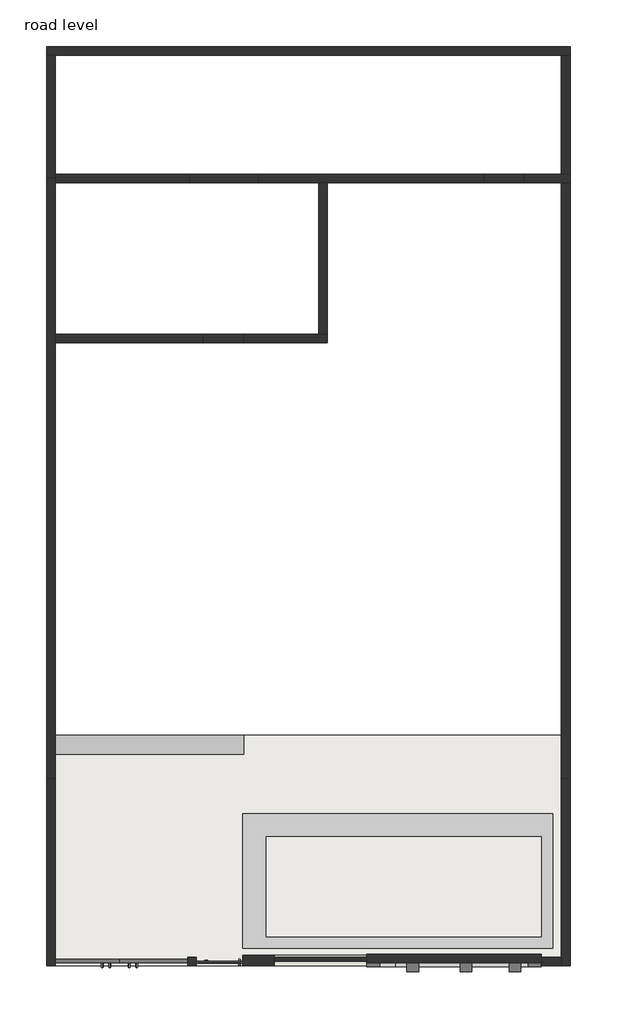
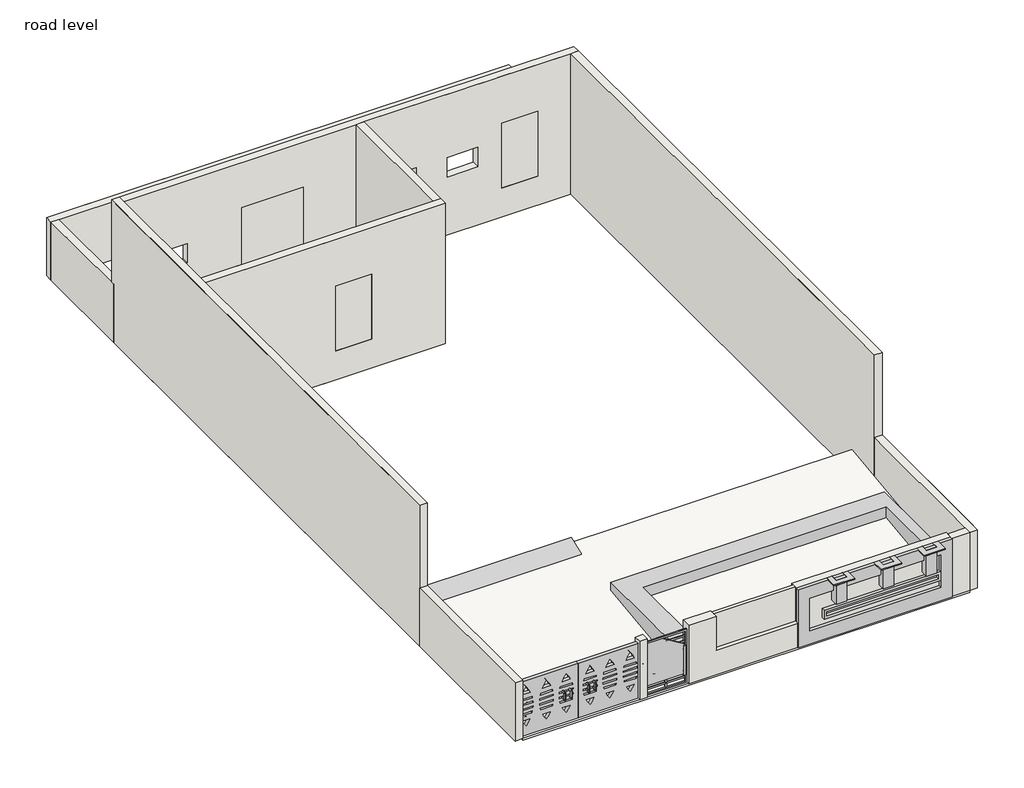
# One storey, incomplete: 28 walls, 5 proxies, 1 slab.
"""IFC4 building model written with IfcOpenShell, lengths in millimetres."""

from ifc_helpers import new_model, si_unit, frame, origin, place, context, project, spatial, polyline, outline, extrude, faceted_brep, transform, mapped, element, save
from components import generic_models_42d6764e, generic_models_918bcdec, generic_models_1_generic_models_1_c1f2a5b8, generic_models_2_generic_models_2_23ebf3b1, generic_models_3_generic_models_3_686a9f3b

model = new_model("IFC4")

# Units and contexts
model_context = context("Model", 3, world=origin())
ifc_project = project(units=[si_unit("LENGTHUNIT", "METRE", prefix="MILLI")], contexts=[model_context])

# Site, building, storey
site = spatial("IfcSite", under=ifc_project)
building = spatial("IfcBuilding", under=site)
storey = spatial("IfcBuildingStorey", under=building, Name="road level", Elevation=-914.4)

# Proxies
placement = place(None, origin())
generic_models_shape = generic_models_42d6764e(model_context)
element("IfcBuildingElementProxy", 1, Name="Generic Models", at=placement, inside=storey, context=model_context, shape_type="MappedRepresentation", body=[
    mapped(generic_models_shape, transform((7221.6695208, -9919.7758122, -914.4), x_axis=(1.0, 0.0, 0.0), y_axis=(0.0, 1.0, 0.0), z_axis=(0.0, 0.0, 1.0))),
])
generic_models_2_shape = generic_models_918bcdec(model_context)
element("IfcBuildingElementProxy", 2, Name="Generic Models", at=placement, inside=storey, context=model_context, shape_type="MappedRepresentation", body=[
    mapped(generic_models_2_shape, transform((10401.6916032, -9983.2758122, -914.4), x_axis=(1.0, 0.0, 0.0), y_axis=(0.0, 1.0, 0.0), z_axis=(0.0, 0.0, 1.0))),
])
generic_models_1_generic_models_1_shape = generic_models_1_generic_models_1_c1f2a5b8(model_context)
element("IfcBuildingElementProxy", 3, Name="Generic Models 1 : Generic Models 1", ObjectType="Generic Models 1 : Generic Models 1", at=placement, inside=storey, context=model_context, shape_type="MappedRepresentation", body=[
    mapped(generic_models_1_generic_models_1_shape, transform((0.0, 0.0, 0.0), x_axis=(1.0, 0.0, 0.0), y_axis=(0.0, 1.0, 0.0), z_axis=(0.0, 0.0, 1.0))),
])
generic_models_2_generic_models_2_shape = generic_models_2_generic_models_2_23ebf3b1(model_context)
element("IfcBuildingElementProxy", 4, Name="Generic Models 2 : Generic Models 2", ObjectType="Generic Models 2 : Generic Models 2", at=placement, inside=storey, context=model_context, shape_type="MappedRepresentation", body=[
    mapped(generic_models_2_generic_models_2_shape, transform((0.0, 0.0, 0.0), x_axis=(1.0, 0.0, 0.0), y_axis=(0.0, 1.0, 0.0), z_axis=(0.0, 0.0, 1.0))),
])
generic_models_3_generic_models_3_shape = generic_models_3_generic_models_3_686a9f3b(model_context)
element("IfcBuildingElementProxy", 5, Name="Generic Models 3 : Generic Models 3", ObjectType="Generic Models 3 : Generic Models 3", at=placement, inside=storey, context=model_context, shape_type="MappedRepresentation", body=[
    mapped(generic_models_3_generic_models_3_shape, transform((0.0, 0.0, 0.0), x_axis=(1.0, 0.0, 0.0), y_axis=(0.0, 1.0, 0.0), z_axis=(0.0, 0.0, 1.0))),
])

# Slab
element("IfcSlab", 6, at=placement, inside=storey, context=model_context, shape_type="SweptSolid", body=[
    extrude(outline(polyline([(-10097.5758122, -965.2), (-10097.5758122, -914.4), (-4052.3758122, -152.4), (-4052.3758122, -203.2), (-10097.5758122, -965.2)])), frame((5486.7916032, 0.0, 0.0), z_axis=(1.0, 0.0, 0.0), x_axis=(0.0, 1.0, 0.0)), (0.0, 0.0, 1.0), 13258.8),
])

# Walls
element("IfcWall", 7, ObjectType="4.5\"", at=placement, inside=storey, context=model_context, shape_type="SweptSolid", body=[
    extrude(outline(polyline([(13640.8433417, -9983.2758122), (11221.8271119, -9983.2758122), (11221.8271119, -9868.9758122), (13640.8433417, -9868.9758122), (13640.8433417, -9983.2758122)])), frame((0.0, 0.0, -914.4), z_axis=(0.0, 0.0, 1.0), x_axis=(1.0, 0.0, 0.0)), (0.0, 0.0, 1.0), 1828.8),
])
element("IfcWall", 8, ObjectType="9\" wall", at=placement, inside=storey, context=model_context, shape_type="SweptSolid", body=[
    extrude(outline(polyline([(5486.7916032, -5195.3758122), (5486.7916032, -10097.5758122), (5258.1916032, -10097.5758122), (5258.1916032, -5195.3758122), (5486.7916032, -5195.3758122)])), frame((0.0, 0.0, -914.4), z_axis=(0.0, 0.0, 1.0), x_axis=(1.0, 0.0, 0.0)), (0.0, 0.0, 1.0), 1828.8),
])
element("IfcWall", 9, ObjectType="9\" wall", at=placement, inside=storey, context=model_context, shape_type="Brep", body=[
    faceted_brep([(5258.1916032, 13753.0241878, -914.4), (5486.7916032, 13753.0241878, -914.4), (18745.5916032, 13753.0241878, -914.4), (18974.1916032, 13753.0241878, -914.4), (18974.1916032, 13753.0241878, 914.4), (18745.5916032, 13753.0241878, 914.4), (5486.7916032, 13753.0241878, 914.4), (5258.1916032, 13753.0241878, 914.4), (5258.1916032, 13981.6241878, -914.4), (5258.1916032, 13981.6241878, 914.4), (18974.1916032, 13981.6241878, 914.4), (18974.1916032, 13981.6241878, -914.4)], [[[0, 1, 2, 3, 4, 5, 6, 7]], [[8, 9, 10, 11]], [[3, 2, 1, 0, 8, 11]], [[7, 6, 5, 4, 10, 9]], [[0, 7, 9, 8]], [[4, 3, 11, 10]]]),
])
element("IfcWall", 10, ObjectType="9\" wall", at=placement, inside=storey, context=model_context, shape_type="Brep", body=[
    faceted_brep([(18745.5916032, -5195.3758122, -914.4), (18745.5916032, -9868.9758122, -914.4), (18745.5916032, -10097.5758122, -914.4), (18745.5916032, -10097.5758122, 914.4), (18745.5916032, -9868.9758122, 914.4), (18745.5916032, -5195.3758122, 914.4), (18974.1916032, -5195.3758122, -914.4), (18974.1916032, -5195.3758122, 914.4), (18974.1916032, -10097.5758122, 914.4), (18974.1916032, -10097.5758122, -914.4)], [[[0, 1, 2, 3, 4, 5]], [[6, 7, 8, 9]], [[2, 1, 0, 6, 9]], [[5, 4, 3, 8, 7]], [[0, 5, 7, 6]], [[3, 2, 9, 8]]]),
])
element("IfcWall", 11, ObjectType="9\" wall", at=placement, inside=storey, context=model_context, shape_type="Brep", body=[
    faceted_brep([(18745.5916032, -9868.9758122, -914.4), (18217.5782182, -9868.9758122, -914.4), (18217.5782182, -9868.9758122, 914.4), (18745.5916032, -9868.9758122, 914.4), (18745.5916032, -10097.5758122, -914.4), (18745.5916032, -10097.5758122, 914.4), (18217.5782182, -10097.5758122, 914.4), (18217.5782182, -10097.5758122, -914.4), (18217.5782182, -10021.3758122, -914.4), (18217.5782182, -10021.3758122, 914.4)], [[[0, 1, 2, 3]], [[4, 5, 6, 7]], [[1, 0, 4, 7, 8]], [[2, 1, 8, 7, 6, 9]], [[3, 2, 9, 6, 5]], [[0, 3, 5, 4]]]),
])
element("IfcWall", 12, ObjectType="9\" wall", at=placement, inside=storey, context=model_context, shape_type="Brep", body=[
    faceted_brep([(18217.5782182, -9792.7758122, -914.4), (13640.8433417, -9792.7758122, -914.4), (13640.8433417, -9792.7758122, 914.4), (18217.5782182, -9792.7758122, 914.4), (18217.5782182, -10021.3758122, -914.4), (18217.5782182, -10021.3758122, 914.4), (13640.8433417, -10021.3758122, 914.4), (13640.8433417, -10021.3758122, -914.4), (18217.5782182, -9868.9758122, -914.4), (13640.8433417, -9983.2758122, -914.4), (13640.8433417, -9868.9758122, -914.4), (13640.8433417, -9818.1758122, -914.4), (13640.8433417, -9868.9758122, 914.4), (13640.8433417, -9983.2758122, 914.4), (18217.5782182, -9868.9758122, 914.4)], [[[0, 1, 2, 3]], [[4, 5, 6, 7]], [[1, 0, 8, 4, 7, 9, 10, 11]], [[3, 2, 12, 13, 6, 5, 14]], [[0, 3, 14, 5, 4, 8]], [[1, 11, 10, 9, 7, 6, 13, 12, 2]]]),
])
element("IfcWall", 13, ObjectType="9\" wall", at=placement, inside=storey, context=model_context, shape_type="Brep", body=[
    faceted_brep([(5258.1916032, 10527.2241878, -914.4), (5258.1916032, -5195.3758122, -914.4), (5258.1916032, -5195.3758122, 914.4), (5258.1916032, -5195.3758122, 3505.2), (5258.1916032, 10641.5241878, 3505.2), (5258.1916032, 10641.5241878, 914.4), (5258.1916032, 10527.2241878, 914.4), (5486.7916032, 10527.2241878, -914.4), (5486.7916032, 10527.2241878, 914.4), (5486.7916032, 10641.5241878, 914.4), (5486.7916032, 10641.5241878, 3505.2), (5486.7916032, 10412.9241878, 3505.2), (5486.7916032, 6450.5241878, 3505.2), (5486.7916032, 6221.9241878, 3505.2), (5486.7916032, 1802.3241878, 3505.2), (5486.7916032, 1573.7241878, 3505.2), (5486.7916032, -5195.3758122, 3505.2), (5486.7916032, -5195.3758122, 914.4), (5486.7916032, -5195.3758122, -914.4), (5486.7916032, 6221.9241878, -914.4), (5486.7916032, 6450.5241878, -914.4), (5486.7916032, 10412.9241878, -914.4)], [[[0, 1, 2, 3, 4, 5, 6]], [[7, 8, 9, 10, 11, 12, 13, 14, 15, 16, 17, 18, 19, 20, 21]], [[1, 0, 7, 21, 20, 19, 18]], [[4, 3, 16, 15, 14, 13, 12, 11, 10]], [[0, 6, 8, 7]], [[5, 9, 8, 6]], [[5, 4, 10, 9]], [[1, 18, 17, 16, 3, 2]]]),
])
element("IfcWall", 14, ObjectType="9\" wall", at=placement, inside=storey, context=model_context, shape_type="Brep", body=[
    faceted_brep([(5258.1916032, 13753.0241878, -914.4), (5258.1916032, 10527.2241878, -914.4), (5258.1916032, 10527.2241878, 914.4), (5258.1916032, 10641.5241878, 914.4), (5258.1916032, 13753.0241878, 914.4), (5486.7916032, 10527.2241878, -914.4), (5486.7916032, 13753.0241878, -914.4), (5486.7916032, 13753.0241878, 914.4), (5486.7916032, 10641.5241878, 914.4), (5486.7916032, 10527.2241878, 914.4)], [[[0, 1, 2, 3, 4]], [[5, 6, 7, 8, 9]], [[1, 0, 6, 5]], [[2, 1, 5, 9]], [[2, 9, 8, 7, 4, 3]], [[0, 4, 7, 6]]]),
])
element("IfcWall", 15, ObjectType="9\" wall", at=placement, inside=storey, context=model_context, shape_type="Brep", body=[
    faceted_brep([(5486.7916032, 10412.9241878, 3505.2), (5486.7916032, 10412.9241878, -914.4), (12382.4099466, 10412.9241878, -914.4), (12611.0099466, 10412.9241878, -914.4), (18745.5916032, 10412.9241878, -914.4), (18974.1916032, 10412.9241878, -914.4), (18974.1916032, 10412.9241878, 3505.2), (18745.5916032, 10412.9241878, 3505.2), (16611.5099466, 10412.9241878, 3505.2), (16497.2099466, 10412.9241878, 3505.2), (12611.0099466, 10412.9241878, 3505.2), (12382.4099466, 10412.9241878, 3505.2), (17773.5599466, 10412.9241878, 0.0), (16706.7599466, 10412.9241878, 0.0), (16706.7599466, 10412.9241878, 2032.0), (17773.5599466, 10412.9241878, 2032.0), (6464.6916032, 10412.9241878, 1524.0), (7379.0916032, 10412.9241878, 1524.0), (7379.0916032, 10412.9241878, 914.4), (6464.6916032, 10412.9241878, 914.4), (14173.1099466, 10412.9241878, 1524.0), (14173.1099466, 10412.9241878, 914.4), (13258.7099466, 10412.9241878, 914.4), (13258.7099466, 10412.9241878, 1524.0), (15081.1599466, 10412.9241878, 1524.0), (15995.5599466, 10412.9241878, 1524.0), (15995.5599466, 10412.9241878, 914.4), (15081.1599466, 10412.9241878, 914.4), (8991.5099466, 10412.9241878, 2082.8), (10820.3099466, 10412.9241878, 2082.8), (10820.3099466, 10412.9241878, 0.0), (8991.5099466, 10412.9241878, 0.0), (5486.7916032, 10641.5241878, -914.4), (5486.7916032, 10641.5241878, 914.4), (5486.7916032, 10641.5241878, 3505.2), (18974.1916032, 10641.5241878, 3505.2), (18974.1916032, 10641.5241878, 914.4), (18974.1916032, 10641.5241878, -914.4), (18745.5916032, 10641.5241878, -914.4), (17773.5599466, 10641.5241878, 0.0), (17773.5599466, 10641.5241878, 2032.0), (16706.7599466, 10641.5241878, 2032.0), (16706.7599466, 10641.5241878, 0.0), (6464.6916032, 10641.5241878, 1524.0), (6464.6916032, 10641.5241878, 914.4), (7379.0916032, 10641.5241878, 914.4), (7379.0916032, 10641.5241878, 1524.0), (14173.1099466, 10641.5241878, 1524.0), (13258.7099466, 10641.5241878, 1524.0), (13258.7099466, 10641.5241878, 914.4), (14173.1099466, 10641.5241878, 914.4), (15081.1599466, 10641.5241878, 1524.0), (15081.1599466, 10641.5241878, 914.4), (15995.5599466, 10641.5241878, 914.4), (15995.5599466, 10641.5241878, 1524.0), (8991.5099466, 10641.5241878, 2082.8), (8991.5099466, 10641.5241878, 0.0), (10820.3099466, 10641.5241878, 0.0), (10820.3099466, 10641.5241878, 2082.8), (5486.7916032, 10527.2241878, -914.4)], [[[0, 1, 2, 3, 4, 5, 6, 7, 8, 9, 10, 11], [12, 13, 14, 15], [16, 17, 18, 19], [20, 21, 22, 23], [24, 25, 26, 27], [28, 29, 30, 31]], [[32, 33, 34, 35, 36, 37, 38], [39, 40, 41, 42], [43, 44, 45, 46], [47, 48, 49, 50], [51, 52, 53, 54], [55, 56, 57, 58]], [[5, 4, 3, 2, 1, 59, 32, 38, 37]], [[0, 11, 10, 9, 8, 7, 6, 35, 34]], [[0, 34, 33, 32, 59, 1]], [[5, 37, 36, 35, 6]], [[13, 12, 39, 42]], [[14, 13, 42, 41]], [[15, 14, 41, 40]], [[12, 15, 40, 39]], [[44, 43, 16, 19]], [[45, 44, 19, 18]], [[46, 45, 18, 17]], [[43, 46, 17, 16]], [[21, 20, 47, 50]], [[22, 21, 50, 49]], [[23, 22, 49, 48]], [[20, 23, 48, 47]], [[52, 51, 24, 27]], [[53, 52, 27, 26]], [[54, 53, 26, 25]], [[51, 54, 25, 24]], [[56, 55, 28, 31]], [[57, 56, 31, 30]], [[58, 57, 30, 29]], [[55, 58, 29, 28]]]),
])
element("IfcWall", 16, ObjectType="9\" wall", at=placement, inside=storey, context=model_context, shape_type="Brep", body=[
    faceted_brep([(18745.5916032, 10412.9241878, 3505.2), (18745.5916032, 10412.9241878, -914.4), (18745.5916032, -5195.3758122, -914.4), (18745.5916032, -5195.3758122, 914.4), (18745.5916032, -5195.3758122, 3505.2), (18745.5916032, -4280.9758122, 3505.2), (18745.5916032, -4052.3758122, 3505.2), (18745.5916032, -699.5758122, 3505.2), (18745.5916032, -585.2758122, 3505.2), (18745.5916032, 1573.7241878, 3505.2), (18745.5916032, 1802.3241878, 3505.2), (18745.5916032, 6221.9241878, 3505.2), (18745.5916032, 6450.5241878, 3505.2), (18974.1916032, 10412.9241878, -914.4), (18974.1916032, 10412.9241878, 3505.2), (18974.1916032, -5195.3758122, 3505.2), (18974.1916032, -5195.3758122, 914.4), (18974.1916032, -5195.3758122, -914.4)], [[[0, 1, 2, 3, 4, 5, 6, 7, 8, 9, 10, 11, 12]], [[13, 14, 15, 16, 17]], [[2, 1, 13, 17]], [[0, 12, 11, 10, 9, 8, 7, 6, 5, 4, 15, 14]], [[0, 14, 13, 1]], [[2, 17, 16, 15, 4, 3]]]),
])
element("IfcWall", 17, ObjectType="9\" wall", at=placement, inside=storey, context=model_context, shape_type="SweptSolid", body=[
    extrude(outline(polyline([(18745.5916032, 10641.5241878), (18745.5916032, 13753.0241878), (18974.1916032, 13753.0241878), (18974.1916032, 10641.5241878), (18745.5916032, 10641.5241878)])), frame((0.0, 0.0, -914.4), z_axis=(0.0, 0.0, 1.0), x_axis=(1.0, 0.0, 0.0)), (0.0, 0.0, 1.0), 1828.8),
])
element("IfcWall", 18, ObjectType="9\" wall", at=placement, inside=storey, context=model_context, shape_type="Brep", body=[
    faceted_brep([(5486.7916032, 6221.9241878, -914.4), (12611.0099466, 6221.9241878, -914.4), (12611.0099466, 6221.9241878, 3505.2), (5486.7916032, 6221.9241878, 3505.2), (10420.2599466, 6221.9241878, 0.0), (9353.4599466, 6221.9241878, 0.0), (9353.4599466, 6221.9241878, 2032.0), (10420.2599466, 6221.9241878, 2032.0), (5486.7916032, 6450.5241878, -914.4), (5486.7916032, 6450.5241878, 3505.2), (7594.5099466, 6450.5241878, 3505.2), (7708.8099466, 6450.5241878, 3505.2), (12382.4099466, 6450.5241878, 3505.2), (12611.0099466, 6450.5241878, 3505.2), (12611.0099466, 6450.5241878, -914.4), (12382.4099466, 6450.5241878, -914.4), (10420.2599466, 6450.5241878, 0.0), (10420.2599466, 6450.5241878, 2032.0), (9353.4599466, 6450.5241878, 2032.0), (9353.4599466, 6450.5241878, 0.0)], [[[0, 1, 2, 3], [4, 5, 6, 7]], [[8, 9, 10, 11, 12, 13, 14, 15], [16, 17, 18, 19]], [[1, 0, 8, 15, 14]], [[3, 2, 13, 12, 11, 10, 9]], [[0, 3, 9, 8]], [[2, 1, 14, 13]], [[5, 4, 16, 19]], [[6, 5, 19, 18]], [[7, 6, 18, 17]], [[4, 7, 17, 16]]]),
])
element("IfcWall", 19, ObjectType="9\" wall", at=placement, inside=storey, context=model_context, shape_type="Brep", body=[
    faceted_brep([(12611.0099466, 6450.5241878, -914.4), (12611.0099466, 10412.9241878, -914.4), (12611.0099466, 10412.9241878, 3505.2), (12611.0099466, 7644.3241878, 3505.2), (12611.0099466, 7530.0241878, 3505.2), (12611.0099466, 6450.5241878, 3505.2), (12382.4099466, 6450.5241878, -914.4), (12382.4099466, 6450.5241878, 3505.2), (12382.4099466, 10412.9241878, 3505.2), (12382.4099466, 10412.9241878, -914.4)], [[[0, 1, 2, 3, 4, 5]], [[6, 7, 8, 9]], [[1, 0, 6, 9]], [[5, 4, 3, 2, 8, 7]], [[0, 5, 7, 6]], [[2, 1, 9, 8]]]),
])
element("IfcWall", 20, ObjectType="9\" wall", at=placement, inside=storey, context=model_context, shape_type="SweptSolid", body=[
    extrude(outline(polyline([(9182.4916032, -10097.5758122), (8953.8916032, -10097.5758122), (8953.8916032, -9868.9758122), (9182.4916032, -9868.9758122), (9182.4916032, -10097.5758122)])), frame((0.0, 0.0, -914.4), z_axis=(0.0, 0.0, 1.0), x_axis=(1.0, 0.0, 0.0)), (0.0, 0.0, 1.0), 1828.8),
])
element("IfcWall", 21, ObjectType="9\" wall", at=placement, inside=storey, context=model_context, shape_type="SweptSolid", body=[
    extrude(outline(polyline([(5486.7916032, -5195.3758122), (5486.7916032, -10097.5758122), (5258.1916032, -10097.5758122), (5258.1916032, -5195.3758122), (5486.7916032, -5195.3758122)])), frame((0.0, 0.0, -914.4), z_axis=(0.0, 0.0, 1.0), x_axis=(1.0, 0.0, 0.0)), (0.0, 0.0, 1.0), 1828.8),
])
element("IfcWall", 22, ObjectType="9\" wall", at=placement, inside=storey, context=model_context, shape_type="SweptSolid", body=[
    extrude(outline(polyline([(18745.5916032, 13753.0241878), (5486.7916032, 13753.0241878), (5486.7916032, 13981.6241878), (18745.5916032, 13981.6241878), (18745.5916032, 13753.0241878)])), frame((0.0, 0.0, -914.4), z_axis=(0.0, 0.0, 1.0), x_axis=(1.0, 0.0, 0.0)), (0.0, 0.0, 1.0), 1828.8),
])
element("IfcWall", 23, ObjectType="9\" wall", at=placement, inside=storey, context=model_context, shape_type="SweptSolid", body=[
    extrude(outline(polyline([(18745.5916032, -9868.9758122), (18745.5916032, -5195.3758122), (18974.1916032, -5195.3758122), (18974.1916032, -9868.9758122), (18745.5916032, -9868.9758122)])), frame((0.0, 0.0, -914.4), z_axis=(0.0, 0.0, 1.0), x_axis=(1.0, 0.0, 0.0)), (0.0, 0.0, 1.0), 1828.8),
])
element("IfcWall", 24, ObjectType="9\" wall", at=placement, inside=storey, context=model_context, shape_type="Brep", body=[
    faceted_brep([(18745.5916032, -9868.9758122, -914.4), (18217.5782182, -9868.9758122, -914.4), (18217.5782182, -9868.9758122, 914.4), (18745.5916032, -9868.9758122, 914.4), (18745.5916032, -10097.5758122, -914.4), (18745.5916032, -10097.5758122, 914.4), (18217.5782182, -10097.5758122, 914.4), (18217.5782182, -10097.5758122, -914.4), (18217.5782182, -10021.3758122, -914.4), (18217.5782182, -10021.3758122, 914.4)], [[[0, 1, 2, 3]], [[4, 5, 6, 7]], [[1, 0, 4, 7, 8]], [[2, 1, 8, 7, 6, 9]], [[3, 2, 9, 6, 5]], [[0, 3, 5, 4]]]),
])
element("IfcWall", 25, ObjectType="9\" wall", at=placement, inside=storey, context=model_context, shape_type="Brep", body=[
    faceted_brep([(18217.5782182, -9792.7758122, -914.4), (13640.8433417, -9792.7758122, -914.4), (13640.8433417, -9792.7758122, 914.4), (18217.5782182, -9792.7758122, 914.4), (18217.5782182, -10021.3758122, -914.4), (18217.5782182, -10021.3758122, 914.4), (13640.8433417, -10021.3758122, 914.4), (13640.8433417, -10021.3758122, -914.4), (18217.5782182, -9868.9758122, -914.4), (18217.5782182, -9868.9758122, 914.4)], [[[0, 1, 2, 3]], [[4, 5, 6, 7]], [[1, 0, 8, 4, 7]], [[3, 2, 6, 5, 9]], [[0, 3, 9, 5, 4, 8]], [[1, 7, 6, 2]]]),
])
element("IfcWall", 26, ObjectType="9\" wall", at=placement, inside=storey, context=model_context, shape_type="Brep", body=[
    faceted_brep([(5258.1916032, 10412.9241878, -914.4), (5258.1916032, -5195.3758122, -914.4), (5258.1916032, -5195.3758122, 914.4), (5258.1916032, -5195.3758122, 3505.2), (5258.1916032, 10412.9241878, 3505.2), (5486.7916032, 10412.9241878, -914.4), (5486.7916032, 10412.9241878, 3505.2), (5486.7916032, 6450.5241878, 3505.2), (5486.7916032, 6221.9241878, 3505.2), (5486.7916032, 1802.3241878, 3505.2), (5486.7916032, 1573.7241878, 3505.2), (5486.7916032, -5195.3758122, 3505.2), (5486.7916032, -5195.3758122, 914.4), (5486.7916032, -5195.3758122, -914.4), (5486.7916032, 6221.9241878, -914.4), (5486.7916032, 6450.5241878, -914.4)], [[[0, 1, 2, 3, 4]], [[5, 6, 7, 8, 9, 10, 11, 12, 13, 14, 15]], [[1, 0, 5, 15, 14, 13]], [[3, 2, 1, 13, 12, 11]], [[4, 3, 11, 10, 9, 8, 7, 6]], [[0, 4, 6, 5]]]),
])
element("IfcWall", 27, ObjectType="9\" wall", at=placement, inside=storey, context=model_context, shape_type="SweptSolid", body=[
    extrude(outline(polyline([(5258.1916032, 10641.5241878), (5258.1916032, 13753.0241878), (5486.7916032, 13753.0241878), (5486.7916032, 10641.5241878), (5258.1916032, 10641.5241878)])), frame((0.0, 0.0, -914.4), z_axis=(0.0, 0.0, 1.0), x_axis=(1.0, 0.0, 0.0)), (0.0, 0.0, 1.0), 1828.8),
])
element("IfcWall", 28, ObjectType="9\" wall", at=placement, inside=storey, context=model_context, shape_type="Brep", body=[
    faceted_brep([(5486.7916032, 10412.9241878, 3505.2), (5486.7916032, 10412.9241878, -914.4), (12382.4099466, 10412.9241878, -914.4), (12611.0099466, 10412.9241878, -914.4), (18745.5916032, 10412.9241878, -914.4), (18745.5916032, 10412.9241878, 3505.2), (12611.0099466, 10412.9241878, 3505.2), (12382.4099466, 10412.9241878, 3505.2), (6464.6916032, 10412.9241878, 1524.0), (7379.0916032, 10412.9241878, 1524.0), (7379.0916032, 10412.9241878, 914.4), (6464.6916032, 10412.9241878, 914.4), (14173.1099466, 10412.9241878, 1524.0), (14173.1099466, 10412.9241878, 914.4), (13258.7099466, 10412.9241878, 914.4), (13258.7099466, 10412.9241878, 1524.0), (15081.1599466, 10412.9241878, 1524.0), (15995.5599466, 10412.9241878, 1524.0), (15995.5599466, 10412.9241878, 914.4), (15081.1599466, 10412.9241878, 914.4), (5486.7916032, 10641.5241878, -914.4), (5486.7916032, 10641.5241878, 914.4), (5486.7916032, 10641.5241878, 3505.2), (18745.5916032, 10641.5241878, 3505.2), (18745.5916032, 10641.5241878, -914.4), (6464.6916032, 10641.5241878, 1524.0), (6464.6916032, 10641.5241878, 914.4), (7379.0916032, 10641.5241878, 914.4), (7379.0916032, 10641.5241878, 1524.0), (14173.1099466, 10641.5241878, 1524.0), (13258.7099466, 10641.5241878, 1524.0), (13258.7099466, 10641.5241878, 914.4), (14173.1099466, 10641.5241878, 914.4), (15081.1599466, 10641.5241878, 1524.0), (15081.1599466, 10641.5241878, 914.4), (15995.5599466, 10641.5241878, 914.4), (15995.5599466, 10641.5241878, 1524.0), (5486.7916032, 10527.2241878, -914.4)], [[[0, 1, 2, 3, 4, 5, 6, 7], [8, 9, 10, 11], [12, 13, 14, 15], [16, 17, 18, 19]], [[20, 21, 22, 23, 24], [25, 26, 27, 28], [29, 30, 31, 32], [33, 34, 35, 36]], [[4, 3, 2, 1, 37, 20, 24]], [[0, 7, 6, 5, 23, 22]], [[26, 25, 8, 11]], [[27, 26, 11, 10]], [[28, 27, 10, 9]], [[25, 28, 9, 8]], [[13, 12, 29, 32]], [[14, 13, 32, 31]], [[15, 14, 31, 30]], [[12, 15, 30, 29]], [[34, 33, 16, 19]], [[35, 34, 19, 18]], [[36, 35, 18, 17]], [[33, 36, 17, 16]], [[0, 22, 21, 20, 37, 1]], [[4, 24, 23, 5]]]),
])
element("IfcWall", 29, ObjectType="9\" wall", at=placement, inside=storey, context=model_context, shape_type="Brep", body=[
    faceted_brep([(18745.5916032, 10412.9241878, 3505.2), (18745.5916032, 10412.9241878, -914.4), (18745.5916032, -5195.3758122, -914.4), (18745.5916032, -5195.3758122, 914.4), (18745.5916032, -5195.3758122, 3505.2), (18745.5916032, -4280.9758122, 3505.2), (18745.5916032, -4052.3758122, 3505.2), (18745.5916032, 1573.7241878, 3505.2), (18745.5916032, 1802.3241878, 3505.2), (18745.5916032, 6221.9241878, 3505.2), (18745.5916032, 6450.5241878, 3505.2), (18974.1916032, 10412.9241878, -914.4), (18974.1916032, 10412.9241878, 3505.2), (18974.1916032, -5195.3758122, 3505.2), (18974.1916032, -5195.3758122, 914.4), (18974.1916032, -5195.3758122, -914.4)], [[[0, 1, 2, 3, 4, 5, 6, 7, 8, 9, 10]], [[11, 12, 13, 14, 15]], [[2, 1, 11, 15]], [[4, 3, 2, 15, 14, 13]], [[0, 10, 9, 8, 7, 6, 5, 4, 13, 12]], [[0, 12, 11, 1]]]),
])
element("IfcWall", 30, ObjectType="9\" wall", at=placement, inside=storey, context=model_context, shape_type="SweptSolid", body=[
    extrude(outline(polyline([(18745.5916032, 10641.5241878), (18745.5916032, 13753.0241878), (18974.1916032, 13753.0241878), (18974.1916032, 10641.5241878), (18745.5916032, 10641.5241878)])), frame((0.0, 0.0, -914.4), z_axis=(0.0, 0.0, 1.0), x_axis=(1.0, 0.0, 0.0)), (0.0, 0.0, 1.0), 1828.8),
])
element("IfcWall", 31, ObjectType="9\" wall", at=placement, inside=storey, context=model_context, shape_type="SweptSolid", body=[
    extrude(outline(polyline([(12382.4099466, 6221.9241878), (5486.7916032, 6221.9241878), (5486.7916032, 6450.5241878), (12382.4099466, 6450.5241878), (12382.4099466, 6221.9241878)])), frame((0.0, 0.0, -914.4), z_axis=(0.0, 0.0, 1.0), x_axis=(1.0, 0.0, 0.0)), (0.0, 0.0, 1.0), 4419.6),
])
element("IfcWall", 32, ObjectType="9\" wall", at=placement, inside=storey, context=model_context, shape_type="SweptSolid", body=[
    extrude(outline(polyline([(12611.0099466, 10412.9241878), (12611.0099466, 6450.5241878), (12382.4099466, 6450.5241878), (12382.4099466, 10412.9241878), (12611.0099466, 10412.9241878)])), frame((0.0, 0.0, -914.4), z_axis=(0.0, 0.0, 1.0), x_axis=(1.0, 0.0, 0.0)), (0.0, 0.0, 1.0), 4419.6),
])
element("IfcWall", 33, ObjectType="9\" wall", at=placement, inside=storey, context=model_context, shape_type="SweptSolid", body=[
    extrude(outline(polyline([(9182.4916032, -10097.5758122), (8953.8916032, -10097.5758122), (8953.8916032, -9868.9758122), (9182.4916032, -9868.9758122), (9182.4916032, -10097.5758122)])), frame((0.0, 0.0, -914.4), z_axis=(0.0, 0.0, 1.0), x_axis=(1.0, 0.0, 0.0)), (0.0, 0.0, 1.0), 1828.8),
])
element("IfcWall", 34, ObjectType="9\" wall 2", at=placement, inside=storey, context=model_context, shape_type="Brep", body=[
    faceted_brep([(11221.8271119, -9818.1758122, -152.4), (13640.8433417, -9818.1758122, -152.4), (13640.8433417, -9818.1758122, -914.4), (10401.6916032, -9818.1758122, -914.4), (10401.6916032, -9818.1758122, 914.4), (11221.8271119, -9818.1758122, 914.4), (11221.8271119, -10097.5758122, -152.4), (11221.8271119, -10097.5758122, 914.4), (10401.6916032, -10097.5758122, 914.4), (10401.6916032, -10097.5758122, -914.4), (13640.8433417, -10097.5758122, -914.4), (13640.8433417, -10097.5758122, -152.4), (13640.8433417, -10021.3758122, -914.4), (11221.8271119, -9983.2758122, 914.4), (11221.8271119, -9868.9758122, 914.4)], [[[0, 1, 2, 3, 4, 5]], [[6, 7, 8, 9, 10, 11]], [[3, 2, 12, 10, 9]], [[4, 3, 9, 8]], [[5, 4, 8, 7, 13, 14]], [[0, 5, 14, 13, 7, 6]], [[1, 0, 6, 11]], [[2, 1, 11, 10, 12]]]),
])

save(model, "model.ifc")

# Revit data of these elements
# Type
#   Default Elevation = 0
# Type
#   sheet = Door - Panel
#   pipe = Door - Panel
#   handal = Door - Panel
#   faram = Door - Panel
#   Default Elevation = 0
# Type
#   Assembly Code = "B1010"
#   Function = 0
#   Layers, outside or top first: 0' - 2" "Wall Material (1)" (function 1)
# Type "4.5\""
#   Assembly Code = "B2010"
#   Layers, outside or top first: 0' - 4 1/2" no material (function 1)
# Type "9\" wall"
#   Assembly Code = "B2010"
#   Layers, outside or top first: 0' - 9" no material (function 1)
# Type "9\" wall 2"
#   Assembly Code = "B2010"
#   Layers, outside or top first: 0' - 2" "Default New Material" (function 4); 0' - 9" "WALL" (function 1)
# Element 1 (IfcBuildingElementProxy)
#   Phase Created = Project Completion
#   Materials on its faces: "GATE"
# Element 2 (IfcBuildingElementProxy)
#   Phase Created = Project Completion
#   Materials on its faces: "Earth", "Door - Panel"
# Element 3 (IfcBuildingElementProxy, "Generic Models 1 : Generic Models 1")
#   Phase Created = A10 - Substructure
# Element 4 (IfcBuildingElementProxy, "Generic Models 2 : Generic Models 2")
#   Phase Created = Project Completion
# Element 5 (IfcBuildingElementProxy, "Generic Models 3 : Generic Models 3")
#   Phase Created = Project Completion
# Element 6 (IfcSlab)
#   Height Offset From Level = 0' - 0"
#   Phase Created = Project Completion
#   Materials on its faces: "Wall Material (1)"
# Element 7 (IfcWall, "4.5\"")
#   Top Offset = 0' - 0"
#   Base Offset = 0' - 0"
#   Unconnected Height = 6' - 0"
#   wall height = 6' - 0"
#   Phase Created = A10 - Substructure
#   Base Constraint = road level
#   Materials on its faces: "Default Wall"
# Elements 8, 9, 10, 11, 12, 14, 17 (IfcWall, "9\" wall")
#   Top Offset = 0' - 0"
#   Base Offset = 0' - 0"
#   Unconnected Height = 6' - 0"
#   wall height = 6' - 0"
#   Phase Created = A10 - Substructure
#   Base Constraint = road level
#   Materials on its faces: "Default Wall"
# Elements 13, 15, 16, 18, 19, 26, 28, 29, 31, 32 (IfcWall, "9\" wall")
#   Top Offset = 0' - 0"
#   Base Offset = 0' - 0"
#   wall height = 14' - 6"
#   Phase Created = Project Completion
#   Base Constraint = road level
#   Top Constraint = FF
#   Materials on its faces: "Default Wall"
# Elements 20, 21, 22, 23, 24, 25, 27, 30, 33 (IfcWall, "9\" wall")
#   Top Offset = 0' - 0"
#   Base Offset = 0' - 0"
#   Unconnected Height = 6' - 0"
#   wall height = 6' - 0"
#   Phase Created = Project Completion
#   Base Constraint = road level
#   Materials on its faces: "Default Wall"
# Element 34 (IfcWall, "9\" wall 2")
#   Top Offset = 0' - 0"
#   Base Offset = 0' - 0"
#   Unconnected Height = 6' - 0"
#   wall height = 6' - 0"
#   Phase Created = A10 - Substructure
#   Base Constraint = road level
#   Materials on its faces: "Default Wall", "WALL", "Default New Material"
# Materials
#   "Door - Panel": class "Wood", colour RGB 210 159 95, transparency 0, Cost = 0
#   "Wall Material (1)": colour RGB 127 127 127, transparency 0, Cost = 0
#   "Default New Material": class "Generic", colour RGB 87 53 23, transparency 0, Cost = 0
#   "WALL": class "Generic", colour RGB 150 150 150, transparency 0, Cost = 0
#   "GATE": class "Generic", colour RGB 120 120 120, transparency 0, Cost = 0
#   "Earth": class "Generic", colour RGB 97 75 62, transparency 0, Description = "Soil", Cost = 0
#   "Default Wall": colour RGB 128 128 128, transparency 0, Cost = 0
